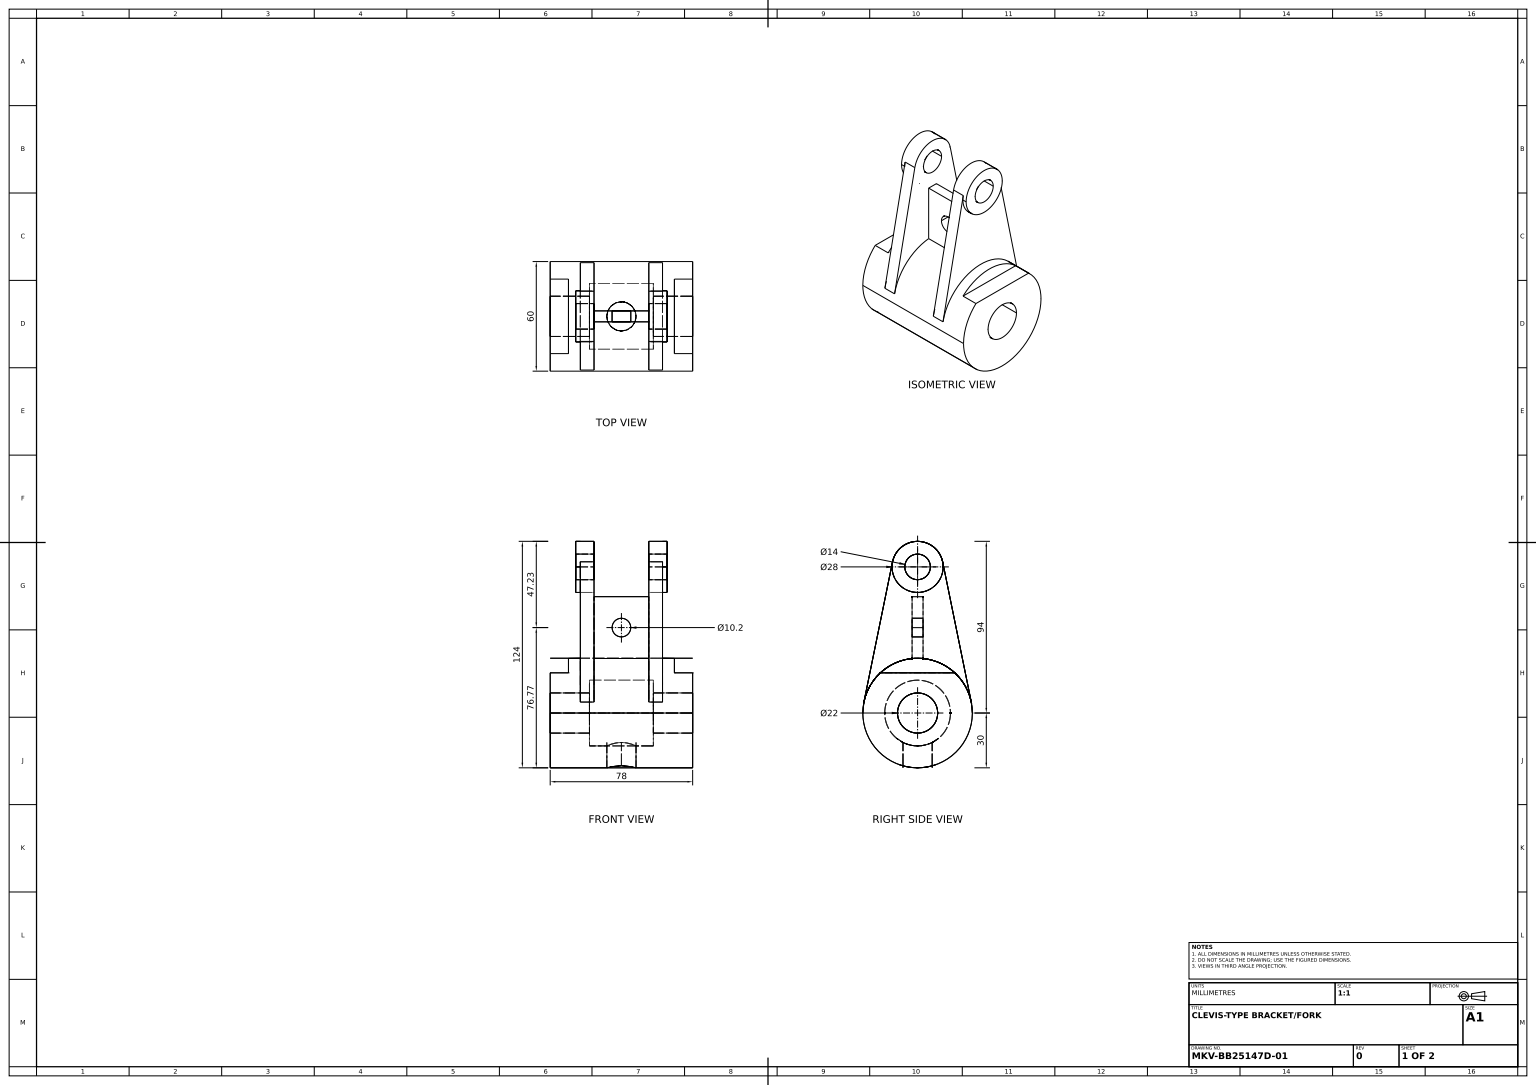
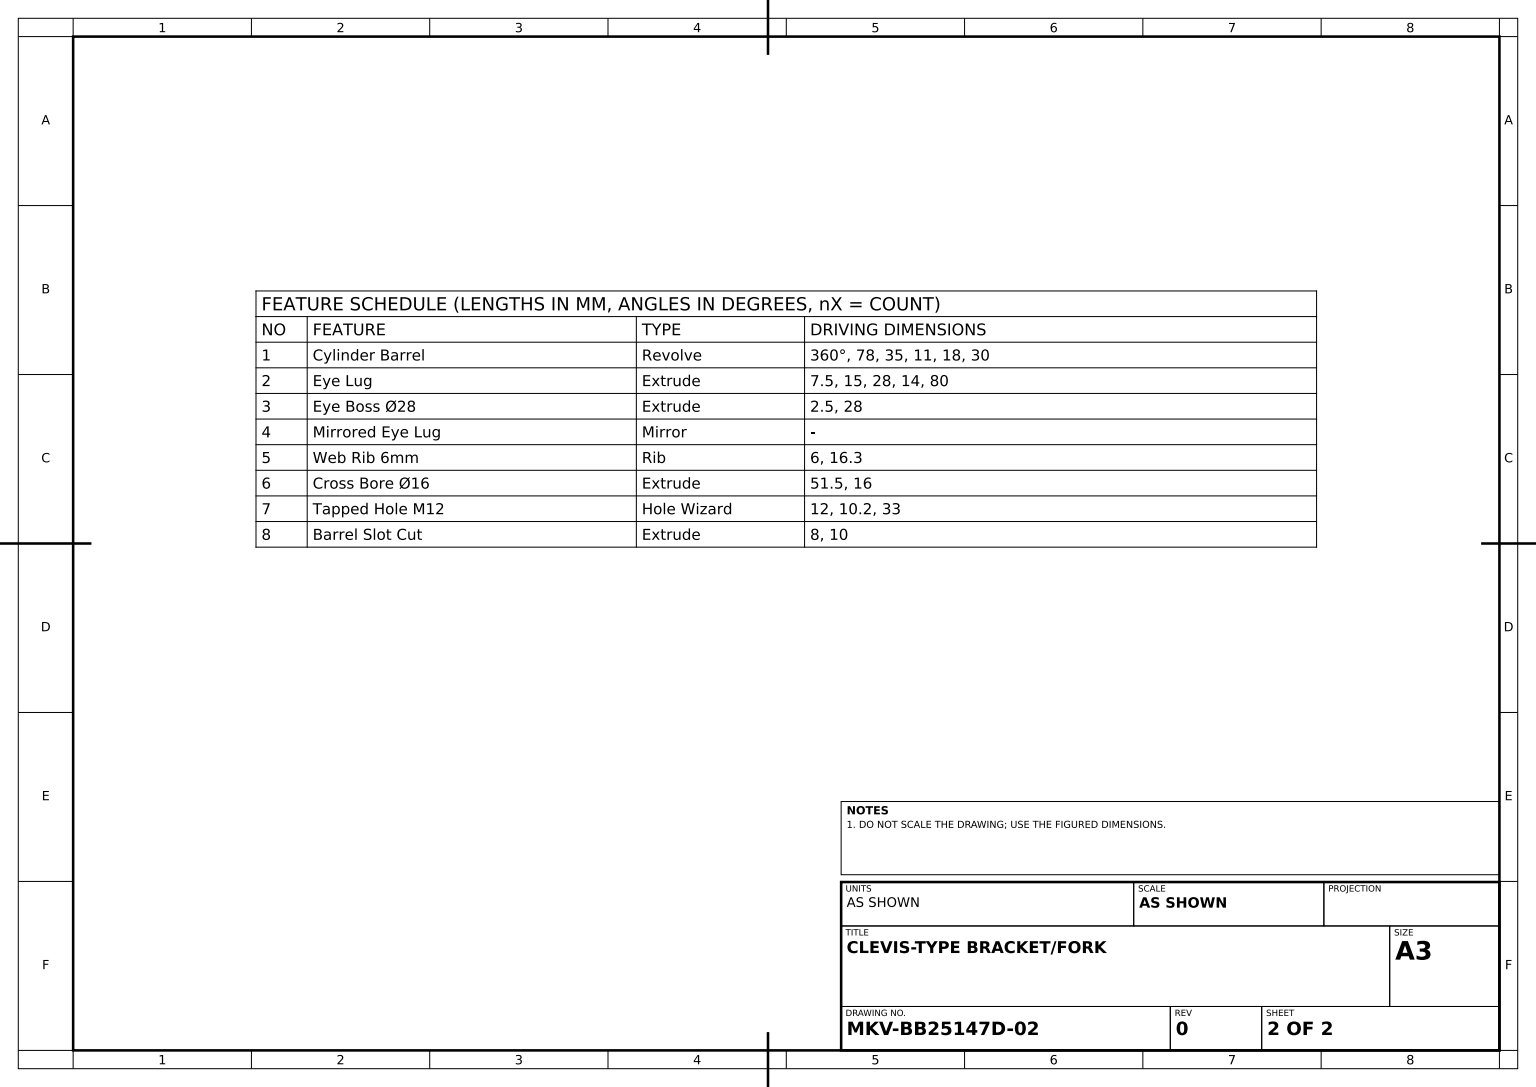
from build123d import *

# Parameters (mm, degrees)
EYE_START                  = 22.5
EYE_LUG_SKETCH_R           = 7
EYE_LUG_DEPTH              = 7.5
EYE_START_2                = 2.5
EYE_BOSS_SKETCH_R          = 14
EYE_BOSS_SKETCH_R_2        = 7
EYE_BOSS_28_DEPTH          = 2.5
WEB_RIB_6MM_REACH          = 108.099
WEB_RIB_SKETCH_WALL_W      = 244.198020726
WEB_RIB_SKETCH_WALL_H      = 6
CROSS_BORE_SKETCH_R        = 8
CROSS_BORE_16_DEPTH        = 51.5
TAPPED_HOLE_M12_D          = 10.2
BARREL_SLOT_CUT_DEPTH      = 107.099010428
BARREL_SLOT_CUT_DEPTH_BACK = 107.099010428
BARREL_SLOT_SKETCH_W       = 10
BARREL_SLOT_SKETCH_H       = 8


with BuildPart() as part:
    # Barrel Profile Sketch → Cylinder Barrel (revolve)
    with BuildSketch(Plane.XY, mode=Mode.PRIVATE) as cylinder_barrel_sk:
        Polygon((-39, 11), (-39, 30), (39, 30), (39, 11), (17.5, 11), (17.5, 18), (-17.5, 18), (-17.5, 11), align=None)
    revolve(cylinder_barrel_sk.sketch.rotate(Axis((-46.634042553, 0, 0), (1, 0, 0)), 90), axis=Axis((-46.634042553, 0, 0), (1, 0, 0)))

    # Eye Lug Sketch → Eye Lug (add)
    with BuildSketch(Plane(origin=(0, 0, 0), x_dir=(0, 0, -1), z_dir=(1, 0, 0)).offset(EYE_START)):
        with BuildLine():
            Line((-29.393876913, 6), (-13.71714256, 82.8))
            ThreePointArc((-13.71714256, 82.8), (0, 94), (13.71714256, 82.8))
            Line((13.71714256, 82.8), (29.393876913, 6))
            ThreePointArc((29.393876913, 6), (0, 30), (-29.393876913, 6))
        make_face()
        with Locations((0, 80)):
            Circle(EYE_LUG_SKETCH_R, mode=Mode.SUBTRACT)
    eye_lug = extrude(amount=-EYE_LUG_DEPTH)

    # Eye Boss Sketch → Eye Boss Ø28 (add)
    with BuildSketch(Plane(origin=(22.5, 0, 0), x_dir=(0, 0, -1), z_dir=(1, 0, 0)).offset(EYE_START_2)):
        with Locations(Location((0, 80, 0), (0, 0, 168.463040967))):
            Circle(EYE_BOSS_SKETCH_R)
        with Locations((0, 80)):
            Circle(EYE_BOSS_SKETCH_R_2, mode=Mode.SUBTRACT)
    eye_boss_28 = extrude(amount=-EYE_BOSS_28_DEPTH)

    # Mirrored Eye Lug: Eye Lug, Eye Boss Ø28 across plane
    add(eye_lug.mirror(Plane(origin=(0, 0, 0), x_dir=(0, 0, 1), z_dir=(1, 0, 0))))
    add(eye_boss_28.mirror(Plane(origin=(0, 0, 0), x_dir=(0, 0, 1), z_dir=(1, 0, 0))))

    # Web Rib Sketch wall → Web Rib 6mm (add, up to next)
    with BuildSketch(Plane(origin=(0, 63.7, 0), x_dir=(1, 0, 0), z_dir=(0, 1, 0)), mode=Mode.PRIVATE) as web_rib_6mm_sk1:
        Rectangle(WEB_RIB_SKETCH_WALL_W, WEB_RIB_SKETCH_WALL_H)
    web_rib_6mm_tool1 = extrude(web_rib_6mm_sk1.sketch, amount=-WEB_RIB_6MM_REACH, mode=Mode.PRIVATE) - part.part
    add(web_rib_6mm_tool1.solids().sort_by_distance((0, 63.7, 0))[0])

    # Cross Bore Sketch → Cross Bore Ø16 (cut)
    with BuildSketch(Plane(origin=(0, 0, 0), x_dir=(1, 0, 0), z_dir=(0, 1, 0))):
        with Locations(Location((0, 0, 0), (0, 0, 270))):
            Circle(CROSS_BORE_SKETCH_R)
    extrude(amount=-CROSS_BORE_16_DEPTH, mode=Mode.SUBTRACT)

    # Tapped Hole M12 (through all)
    with Locations(Plane(origin=(0, 46.774811557, 3), x_dir=(1, 0, 0), z_dir=(0, 0, 1))):
        with Locations((0, 0)):
            Hole(TAPPED_HOLE_M12_D / 2)

    # Barrel Slot Sketch → Barrel Slot Cut (cut, two sides: drawn at the far end of the back side and taken through both)
    with BuildSketch(Plane.XY.offset(-BARREL_SLOT_CUT_DEPTH_BACK)):
        with Locations((-34, 26)):
            Rectangle(BARREL_SLOT_SKETCH_W, BARREL_SLOT_SKETCH_H)
        with Locations((34, 26)):
            Rectangle(BARREL_SLOT_SKETCH_W, BARREL_SLOT_SKETCH_H)
    extrude(amount=BARREL_SLOT_CUT_DEPTH + BARREL_SLOT_CUT_DEPTH_BACK, mode=Mode.SUBTRACT)


solid = part.part
